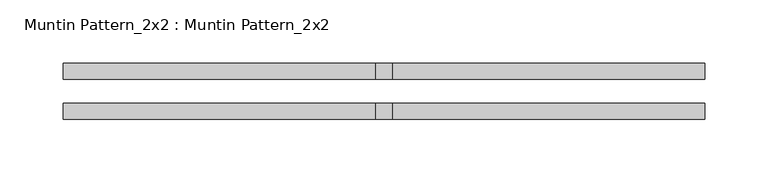
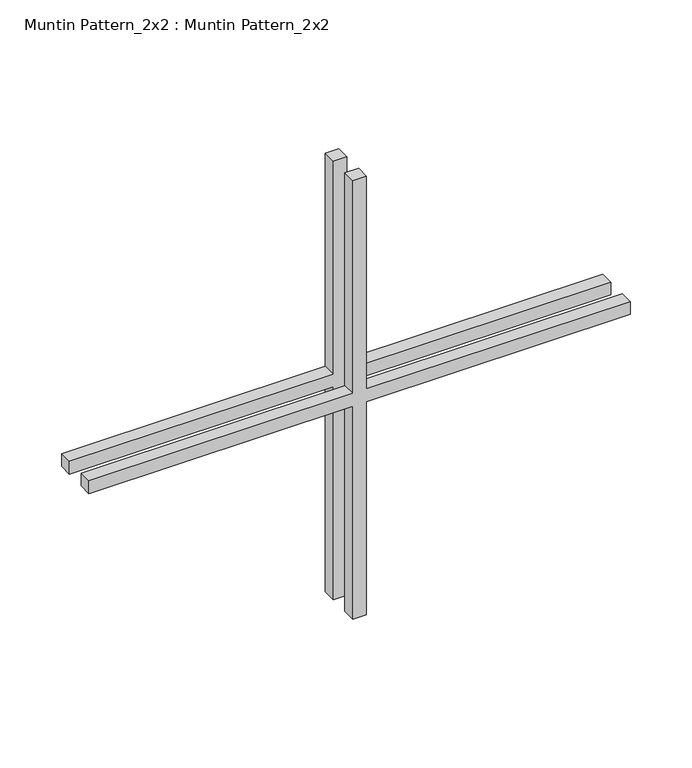
"""IFC4 building model written with IfcOpenShell, lengths in millimetres: proxy geometry, Muntin Pattern_2x2 : Muntin Pattern_2x2."""

from ifc_helpers import new_model, si_unit, frame, origin, place, context, project, spatial, polyline, outline, extrude, source, transform, mapped, element, save


def muntin_pattern_2x2_muntin_pattern_2x2_c35c595f(model_context):
    return source(origin(), model_context, "Body", "SweptSolid", [
        extrude(outline(polyline([(223.8375, -6.35), (223.8375, -254.0), (211.1375, -254.0), (211.1375, -6.35), (0.0, -6.35), (0.0, 6.35), (211.1375, 6.35), (211.1375, 254.0), (223.8375, 254.0), (223.8375, 6.35), (434.975, 6.35), (434.975, -6.35), (223.8375, -6.35)])), frame((0.0, 9.525, 0.0), z_axis=(0.0, 1.0, 0.0), x_axis=(0.0, 0.0, 1.0)), (0.0, 0.0, 1.0), 12.7),
        extrude(outline(polyline([(223.8375, -6.35), (223.8375, -254.0), (211.1375, -254.0), (211.1375, -6.35), (0.0, -6.35), (0.0, 6.35), (211.1375, 6.35), (211.1375, 254.0), (223.8375, 254.0), (223.8375, 6.35), (434.975, 6.35), (434.975, -6.35), (223.8375, -6.35)])), frame((0.0, -22.225, 0.0), z_axis=(0.0, 1.0, 0.0), x_axis=(0.0, 0.0, 1.0)), (0.0, 0.0, 1.0), 12.7),
    ])


if __name__ == "__main__":
    model = new_model("IFC4")
    model_context = context("Model", 3, world=origin())
    ifc_project = project(units=[si_unit("LENGTHUNIT", "METRE", prefix="MILLI")], contexts=[model_context])
    site = spatial("IfcSite", under=ifc_project)
    building = spatial("IfcBuilding", under=site)
    placement = place(None, origin())
    muntin_pattern_2x2_muntin_pattern_2x2_shape = muntin_pattern_2x2_muntin_pattern_2x2_c35c595f(model_context)
    element("IfcBuildingElementProxy", 1, Name="Muntin Pattern_2x2 : Muntin Pattern_2x2", ObjectType="Muntin Pattern_2x2 : Muntin Pattern_2x2", at=placement, inside=building, context=model_context, shape_type="MappedRepresentation", body=[
        mapped(muntin_pattern_2x2_muntin_pattern_2x2_shape, transform((0.0, 0.0, 0.0), x_axis=(1.0, 0.0, 0.0), y_axis=(0.0, 1.0, 0.0), z_axis=(0.0, 0.0, 1.0))),
    ])
    save(model, "model.ifc")

# Revit data of these elements
# Type "Muntin Pattern_2x2 : Muntin Pattern_2x2"
#   Width [instance default] = 4' - 0"
#   Thickness = 0' - 0 1/2"
#   Height [instance default] = 4' - 0"
#   Distance = 0' - 0 3/4"
#   Interior Material [instance default] = none
#   Exterior Material [instance default] = none
#   Default Elevation = 0
# Element 1 (IfcBuildingElementProxy, "Muntin Pattern_2x2 : Muntin Pattern_2x2")
#   Width = 1' - 8"
#   Height = 1' - 5 1/8"
#   Interior Material = Wood - Stained
#   Exterior Material = Clad - White
#   Materials on its faces: "Clad - White", "Wood - Stained"
# Materials
#   "Clad - White": class "Wood", colour RGB 242 242 238, transparency 0, Cost = 0
#   "Wood - Stained": class "Wood", colour RGB 224 178 126, transparency 0, Cost = 0
